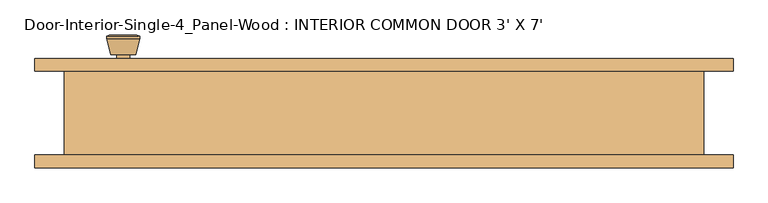
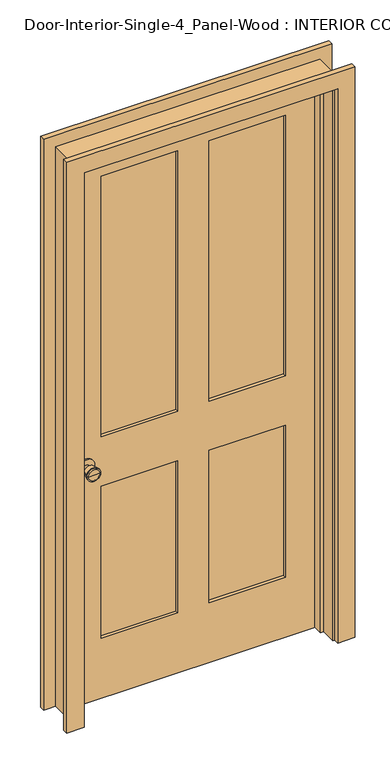
"""IFC4 building model written with IfcOpenShell, lengths in millimetres: door geometry, Door-Interior-Single-4_Panel-Wood : INTERIOR COMMON DOOR 3' X 7'."""

from ifc_helpers import new_model, si_unit, point, frame, frame_2d, origin, place, context, project, spatial, polyline, circle_curve, trimmed, segment, composite_curve, outline, extrude, faceted_brep, source, transform, mapped, element, save
from ifc_brep_helpers import plane_surface, cylinder_surface, revolved_surface, advanced_brep


def door_interior_single_4_panel_wood_interior_common_door_3_x_7_68a706ac(model_context):
    return source(origin(), model_context, "Body", "SolidModel", [
        advanced_brep(
        [(-393.7, 19.4, 914.4), (-383.7, 19.4, 914.4), (-403.7, 19.4, 914.4), (-373.2241324, -29.6, 914.4), (-393.7, -29.6, 914.4), (-414.1758676, -29.6, 914.4), (-368.7, -27.7721319, 914.4), (-418.7, -27.7721319, 914.4), (-368.7, -24.3084537, 914.4), (-418.7, -24.3084537, 914.4), (-375.063764, 0.4, 914.4), (-412.336236, 0.4, 914.4), (-383.7, 0.4, 914.4), (-403.7, 0.4, 914.4)],
        [
            (0, 1),
            (1, 2, circle_curve(frame((-393.7, 19.4, 914.4), z_axis=(0.0, 1.0, 0.0), x_axis=(-1.0, 0.0, 0.0)), 10.0)),
            (2, 0),
            (2, 1, circle_curve(frame((-393.7, 19.4, 914.4), z_axis=(0.0, 1.0, 0.0), x_axis=(-1.0, 0.0, 0.0)), 10.0)),
            (3, 4),
            (4, 5),
            (5, 3, circle_curve(frame((-393.7, -29.6, 914.4), z_axis=(0.0, -1.0, 0.0), x_axis=(-1.0, 0.0, 0.0)), 20.4758676)),
            (3, 5, circle_curve(frame((-393.7, -29.6, 914.4), z_axis=(0.0, -1.0, 0.0), x_axis=(-1.0, 0.0, 0.0)), 20.4758676)),
            (6, 3),
            (5, 7),
            (7, 6, circle_curve(frame((-393.7, -27.7721319, 914.4), z_axis=(0.0, -1.0, 0.0), x_axis=(-1.0, 0.0, 0.0)), 25.0)),
            (6, 7, circle_curve(frame((-393.7, -27.7721319, 914.4), z_axis=(0.0, -1.0, 0.0), x_axis=(-1.0, 0.0, 0.0)), 25.0)),
            (8, 6),
            (7, 9),
            (9, 8, circle_curve(frame((-393.7, -24.3084537, 914.4), z_axis=(0.0, -1.0, 0.0), x_axis=(-1.0, 0.0, 0.0)), 25.0)),
            (8, 9, circle_curve(frame((-393.7, -24.3084537, 914.4), z_axis=(0.0, -1.0, 0.0), x_axis=(-1.0, 0.0, 0.0)), 25.0)),
            (10, 8),
            (9, 11),
            (11, 10, circle_curve(frame((-393.7, 0.4, 914.4), z_axis=(0.0, -1.0, 0.0), x_axis=(-1.0, 0.0, 0.0)), 18.636236)),
            (10, 11, circle_curve(frame((-393.7, 0.4, 914.4), z_axis=(0.0, -1.0, 0.0), x_axis=(-1.0, 0.0, 0.0)), 18.636236)),
            (12, 10),
            (11, 13),
            (13, 12, circle_curve(frame((-393.7, 0.4, 914.4), z_axis=(0.0, -1.0, 0.0), x_axis=(-1.0, 0.0, 0.0)), 10.0)),
            (12, 13, circle_curve(frame((-393.7, 0.4, 914.4), z_axis=(0.0, -1.0, 0.0), x_axis=(-1.0, 0.0, 0.0)), 10.0)),
            (1, 12),
            (13, 2),
        ],
        [
            plane_surface(frame((-393.7, 19.4, 914.4), z_axis=(0.0, 1.0, 0.0), x_axis=(-1.0, 0.0, 0.0))),
            plane_surface(frame((-393.7, -29.6, 914.4), z_axis=(0.0, -1.0, 0.0), x_axis=(-1.0, 0.0, 0.0))),
            revolved_surface(polyline([(-414.1758676, -29.6, 914.4), (-418.7, -27.7721319, 914.4)]), (-393.7, 19.4, 914.4), (0.0, 1.0, 0.0)),
            cylinder_surface(frame((-393.7, 19.4, 914.4), z_axis=(0.0, 1.0, 0.0), x_axis=(-1.0, 0.0, 0.0)), 25.0),
            revolved_surface(polyline([(-418.7, -24.3084537, 914.4), (-412.336236, 0.4, 914.4)]), (-393.7, 19.4, 914.4), (0.0, 1.0, 0.0)),
            plane_surface(frame((-393.7, 0.4, 914.4), z_axis=(0.0, 1.0, 0.0), x_axis=(-1.0, 0.0, 0.0))),
            cylinder_surface(frame((-393.7, 19.4, 914.4), z_axis=(0.0, 1.0, 0.0), x_axis=(-1.0, 0.0, 0.0)), 10.0),
        ],
        [
            (0, [[1, 2, 3]]),
            (0, [[-3, 4, -1]]),
            (1, [[5, 6, 7]]),
            (1, [[-6, -5, 8]]),
            (2, [[9, -7, 10, 11]]),
            (2, [[-10, -8, -9, 12]]),
            (3, [[13, -11, 14, 15]]),
            (3, [[-14, -12, -13, 16]]),
            (4, [[17, -15, 18, 19]]),
            (4, [[-18, -16, -17, 20]]),
            (5, [[21, -19, 22, 23]]),
            (5, [[-22, -20, -21, 24]]),
            (6, [[25, -23, 26, -2]]),
            (6, [[-26, -24, -25, -4]]),
        ],
    ),
        extrude(outline(composite_curve([segment(trimmed(circle_curve(frame_2d((914.4, -393.7)), 30.0), [point((914.4, -423.7))], [point((914.4, -363.7))], False, "CARTESIAN"), True, "CONTINUOUS"), segment(trimmed(circle_curve(frame_2d((914.4, -393.7)), 30.0), [point((914.4, -363.7))], [point((914.4, -423.7))], False, "CARTESIAN"), True, "CONTINUOUS")], self_intersect=False)), frame((0.0, 19.4, 0.0), z_axis=(0.0, 1.0, 0.0), x_axis=(0.0, 0.0, 1.0)), (0.0, 0.0, 1.0), 6.0),
        advanced_brep(
        [(-393.7, 66.325, 914.4), (-403.7, 66.325, 914.4), (-383.7, 66.325, 914.4), (-373.2241324, 115.325, 914.4), (-414.1758676, 115.325, 914.4), (-393.7, 115.325, 914.4), (-368.7, 113.4971319, 914.4), (-418.7, 113.4971319, 914.4), (-368.7, 110.0334537, 914.4), (-418.7, 110.0334537, 914.4), (-375.063764, 85.325, 914.4), (-412.336236, 85.325, 914.4), (-383.7, 85.325, 914.4), (-403.7, 85.325, 914.4)],
        [
            (0, 1),
            (1, 2, circle_curve(frame((-393.7, 66.325, 914.4), z_axis=(0.0, -1.0, 0.0), x_axis=(-1.0, 0.0, 0.0)), 10.0)),
            (2, 0),
            (2, 1, circle_curve(frame((-393.7, 66.325, 914.4), z_axis=(0.0, -1.0, 0.0), x_axis=(-1.0, 0.0, 0.0)), 10.0)),
            (3, 4, circle_curve(frame((-393.7, 115.325, 914.4), z_axis=(0.0, 1.0, 0.0), x_axis=(-1.0, 0.0, 0.0)), 20.4758676)),
            (4, 5),
            (5, 3),
            (4, 3, circle_curve(frame((-393.7, 115.325, 914.4), z_axis=(0.0, 1.0, 0.0), x_axis=(-1.0, 0.0, 0.0)), 20.4758676)),
            (6, 7, circle_curve(frame((-393.7, 113.4971319, 914.4), z_axis=(0.0, 1.0, 0.0), x_axis=(-1.0, 0.0, 0.0)), 25.0)),
            (7, 4),
            (3, 6),
            (7, 6, circle_curve(frame((-393.7, 113.4971319, 914.4), z_axis=(0.0, 1.0, 0.0), x_axis=(-1.0, 0.0, 0.0)), 25.0)),
            (8, 9, circle_curve(frame((-393.7, 110.0334537, 914.4), z_axis=(0.0, 1.0, 0.0), x_axis=(-1.0, 0.0, 0.0)), 25.0)),
            (9, 7),
            (6, 8),
            (9, 8, circle_curve(frame((-393.7, 110.0334537, 914.4), z_axis=(0.0, 1.0, 0.0), x_axis=(-1.0, 0.0, 0.0)), 25.0)),
            (10, 11, circle_curve(frame((-393.7, 85.325, 914.4), z_axis=(0.0, 1.0, 0.0), x_axis=(-1.0, 0.0, 0.0)), 18.636236)),
            (11, 9),
            (8, 10),
            (11, 10, circle_curve(frame((-393.7, 85.325, 914.4), z_axis=(0.0, 1.0, 0.0), x_axis=(-1.0, 0.0, 0.0)), 18.636236)),
            (12, 13, circle_curve(frame((-393.7, 85.325, 914.4), z_axis=(0.0, 1.0, 0.0), x_axis=(-1.0, 0.0, 0.0)), 10.0)),
            (13, 11),
            (10, 12),
            (13, 12, circle_curve(frame((-393.7, 85.325, 914.4), z_axis=(0.0, 1.0, 0.0), x_axis=(-1.0, 0.0, 0.0)), 10.0)),
            (1, 13),
            (12, 2),
        ],
        [
            plane_surface(frame((-393.7, 66.325, 914.4), z_axis=(0.0, -1.0, 0.0), x_axis=(-1.0, 0.0, 0.0))),
            plane_surface(frame((-393.7, 115.325, 914.4), z_axis=(0.0, 1.0, 0.0), x_axis=(-1.0, 0.0, 0.0))),
            revolved_surface(polyline([(-414.1758676, 115.325, 914.4), (-418.7, 113.4971319, 914.4)]), (-393.7, 66.325, 914.4), (0.0, -1.0, 0.0)),
            cylinder_surface(frame((-393.7, 66.325, 914.4), z_axis=(0.0, -1.0, 0.0), x_axis=(-1.0, 0.0, 0.0)), 25.0),
            revolved_surface(polyline([(-418.7, 110.0334537, 914.4), (-412.336236, 85.325, 914.4)]), (-393.7, 66.325, 914.4), (0.0, -1.0, 0.0)),
            plane_surface(frame((-393.7, 85.325, 914.4), z_axis=(0.0, -1.0, 0.0), x_axis=(-1.0, 0.0, 0.0))),
            cylinder_surface(frame((-393.7, 66.325, 914.4), z_axis=(0.0, -1.0, 0.0), x_axis=(-1.0, 0.0, 0.0)), 10.0),
        ],
        [
            (0, [[1, 2, 3]]),
            (0, [[-3, 4, -1]]),
            (1, [[5, 6, 7]]),
            (1, [[8, -7, -6]]),
            (2, [[9, 10, -5, 11]]),
            (2, [[12, -11, -8, -10]]),
            (3, [[13, 14, -9, 15]]),
            (3, [[16, -15, -12, -14]]),
            (4, [[17, 18, -13, 19]]),
            (4, [[20, -19, -16, -18]]),
            (5, [[21, 22, -17, 23]]),
            (5, [[24, -23, -20, -22]]),
            (6, [[-2, 25, -21, 26]]),
            (6, [[-4, -26, -24, -25]]),
        ],
    ),
        extrude(outline(composite_curve([segment(trimmed(circle_curve(frame_2d((914.4, -393.7)), 30.0), [point((914.4, -423.7))], [point((914.4, -363.7))], False, "CARTESIAN"), True, "CONTINUOUS"), segment(trimmed(circle_curve(frame_2d((914.4, -393.7)), 30.0), [point((914.4, -363.7))], [point((914.4, -423.7))], False, "CARTESIAN"), True, "CONTINUOUS")], self_intersect=False)), frame((0.0, 60.325, 0.0), z_axis=(0.0, 1.0, 0.0), x_axis=(0.0, 0.0, 1.0)), (0.0, 0.0, 1.0), 6.0),
        faceted_brep([(482.6, 60.325, 0.0), (482.6, -66.675, 0.0), (457.2, -66.675, 0.0), (457.2, -9.525, 0.0), (444.5, -9.525, 0.0), (444.5, 25.4, 0.0), (457.2, 25.4, 0.0), (457.2, 60.325, 0.0), (482.6, 60.325, 2159.0), (482.6, -66.675, 2159.0), (-482.6, -66.675, 2159.0), (-482.6, -66.675, 0.0), (-457.2, -66.675, 0.0), (-457.2, -66.675, 2133.6), (457.2, -66.675, 2133.6), (457.2, -9.525, 2133.6), (-457.2, -9.525, 2133.6), (-457.2, -9.525, 0.0), (-444.5, -9.525, 0.0), (-444.5, -9.525, 2120.9), (444.5, -9.525, 2120.9), (444.5, 25.4, 2120.9), (-444.5, 25.4, 2120.9), (-444.5, 25.4, 0.0), (-457.2, 25.4, 0.0), (-457.2, 25.4, 2133.6), (457.2, 25.4, 2133.6), (457.2, 60.325, 2133.6), (-457.2, 60.325, 2133.6), (-457.2, 60.325, 0.0), (-482.6, 60.325, 0.0), (-482.6, 60.325, 2159.0)], [[[0, 1, 2, 3, 4, 5, 6, 7]], [[1, 0, 8, 9]], [[2, 1, 9, 10, 11, 12, 13, 14]], [[3, 2, 14, 15]], [[4, 3, 15, 16, 17, 18, 19, 20]], [[5, 4, 20, 21]], [[6, 5, 21, 22, 23, 24, 25, 26]], [[7, 6, 26, 27]], [[0, 7, 27, 28, 29, 30, 31, 8]], [[9, 8, 31, 10]], [[15, 14, 13, 16]], [[21, 20, 19, 22]], [[27, 26, 25, 28]], [[30, 29, 24, 23, 18, 17, 12, 11]], [[10, 31, 30, 11]], [[16, 13, 12, 17]], [[22, 19, 18, 23]], [[28, 25, 24, 29]]]),
        extrude(outline(polyline([(2133.6, -457.2), (0.0, -457.2), (0.0, 457.2), (2133.6, 457.2), (2133.6, -457.2)]), holes=[polyline([(2014.5375, 57.15), (2014.5375, 336.55), (1009.65, 336.55), (1009.65, 57.15), (2014.5375, 57.15)]), polyline([(1009.65, -57.15), (1009.65, -336.55), (2014.5375, -336.55), (2014.5375, -57.15), (1009.65, -57.15)]), polyline([(819.15, 57.15), (819.15, 336.55), (231.775, 336.55), (231.775, 57.15), (819.15, 57.15)]), polyline([(231.775, -57.15), (231.775, -336.55), (819.15, -336.55), (819.15, -57.15), (231.775, -57.15)])]), frame((0.0, 25.4, 0.0), z_axis=(0.0, 1.0, 0.0), x_axis=(0.0, 0.0, 1.0)), (0.0, 0.0, 1.0), 34.925),
        extrude(outline(polyline([(336.55, 37.0416667), (57.15, 37.0416667), (57.15, 48.6833333), (336.55, 48.6833333), (336.55, 37.0416667)])), frame((0.0, 0.0, 1009.65), z_axis=(0.0, 0.0, 1.0), x_axis=(1.0, 0.0, 0.0)), (0.0, 0.0, 1.0), 1004.8875),
        extrude(outline(polyline([(-57.15, 37.0416667), (-336.55, 37.0416667), (-336.55, 48.6833333), (-57.15, 48.6833333), (-57.15, 37.0416667)])), frame((0.0, 0.0, 1009.65), z_axis=(0.0, 0.0, 1.0), x_axis=(1.0, 0.0, 0.0)), (0.0, 0.0, 1.0), 1004.8875),
        extrude(outline(polyline([(336.55, 37.0416667), (57.15, 37.0416667), (57.15, 48.6833333), (336.55, 48.6833333), (336.55, 37.0416667)])), frame((0.0, 0.0, 231.775), z_axis=(0.0, 0.0, 1.0), x_axis=(1.0, 0.0, 0.0)), (0.0, 0.0, 1.0), 587.375),
        extrude(outline(polyline([(-57.15, 37.0416667), (-336.55, 37.0416667), (-336.55, 48.6833333), (-57.15, 48.6833333), (-57.15, 37.0416667)])), frame((0.0, 0.0, 231.775), z_axis=(0.0, 0.0, 1.0), x_axis=(1.0, 0.0, 0.0)), (0.0, 0.0, 1.0), 587.375),
        extrude(outline(polyline([(0.0, 463.55), (0.0, 527.05), (2203.45, 527.05), (2203.45, -527.05), (0.0, -527.05), (0.0, -463.55), (2139.95, -463.55), (2139.95, 463.55), (0.0, 463.55)])), frame((0.0, 60.325, 0.0), z_axis=(0.0, 1.0, 0.0), x_axis=(0.0, 0.0, 1.0)), (0.0, 0.0, 1.0), 19.05),
        extrude(outline(polyline([(0.0, 463.55), (0.0, 527.05), (2203.45, 527.05), (2203.45, -527.05), (0.0, -527.05), (0.0, -463.55), (2139.95, -463.55), (2139.95, 463.55), (0.0, 463.55)])), frame((0.0, -85.725, 0.0), z_axis=(0.0, 1.0, 0.0), x_axis=(0.0, 0.0, 1.0)), (0.0, 0.0, 1.0), 19.05),
    ])


if __name__ == "__main__":
    model = new_model("IFC4")
    model_context = context("Model", 3, world=origin())
    ifc_project = project(units=[si_unit("LENGTHUNIT", "METRE", prefix="MILLI")], contexts=[model_context])
    site = spatial("IfcSite", under=ifc_project)
    building = spatial("IfcBuilding", under=site)
    placement = place(None, origin())
    door_interior_single_4_panel_wood_interior_common_door_3_x_7_shape = door_interior_single_4_panel_wood_interior_common_door_3_x_7_68a706ac(model_context)
    element("IfcDoor", 1, ObjectType="Door-Interior-Single-4_Panel-Wood : INTERIOR COMMON DOOR 3' X 7'", at=placement, inside=building, context=model_context, shape_type="MappedRepresentation", body=[
        mapped(door_interior_single_4_panel_wood_interior_common_door_3_x_7_shape, transform((0.0, 0.0, 0.0), x_axis=(1.0, 0.0, 0.0), y_axis=(0.0, 1.0, 0.0), z_axis=(0.0, 0.0, 1.0))),
    ])
    save(model, "model.ifc")

# Revit data of these elements
# Type "Door-Interior-Single-4_Panel-Wood : INTERIOR COMMON DOOR 3' X 7'"
#   Type Mark = "11"
#   Assembly Code = "C1020300"
#   Analytic Construction = "Wooden"
#   Top Rail = 0' - 4 11/16"
#   Thickness = 0' - 1 3/8"
#   Thermal Resistance (R) = 2.5876 (h·ft²·°F)/BTU
#   Swing Angle [instance default] = 90.00°
#   Stiles = 0' - 4 3/4"
#   Rough Width = 3' - 2"
#   Rough Height = 7' - 1"
#   Mullion = 0' - 4 1/2"
#   Lock Rail = 0' - 7 1/2"
#   Height = 7' - 0"
#   Width = 3' - 0"
#   Heat Transfer Coefficient (U) = 0.3865 BTU/(h·ft²·°F)
#   Bottom Rail = 0' - 9 1/8"
#   Trim Material = Cherry
#   Panel Material = Cherry
#   Frame Material = Cherry
#   Door Handle Material = Aluminum
#   Visual Light Transmittance = 0
#   Solar Heat Gain Coefficient = 0
#   Wall Closure = (empty or 0)
#   Function = (empty or 0)
# Element 1 (IfcDoor, "Door-Interior-Single-4_Panel-Wood : INTERIOR COMMON DOOR 3' X 7'")
#   Materials on its faces: "Cherry", "Aluminum"
# Materials
#   "Cherry": class "Wood", colour RGB 226 177 128, transparency 0, Description = "Prunus Serotina", Cost = 0
#   "Aluminum": class "Metal", colour RGB 247 247 247, transparency 0, Description = "Aluminum 6061", Cost = 0
